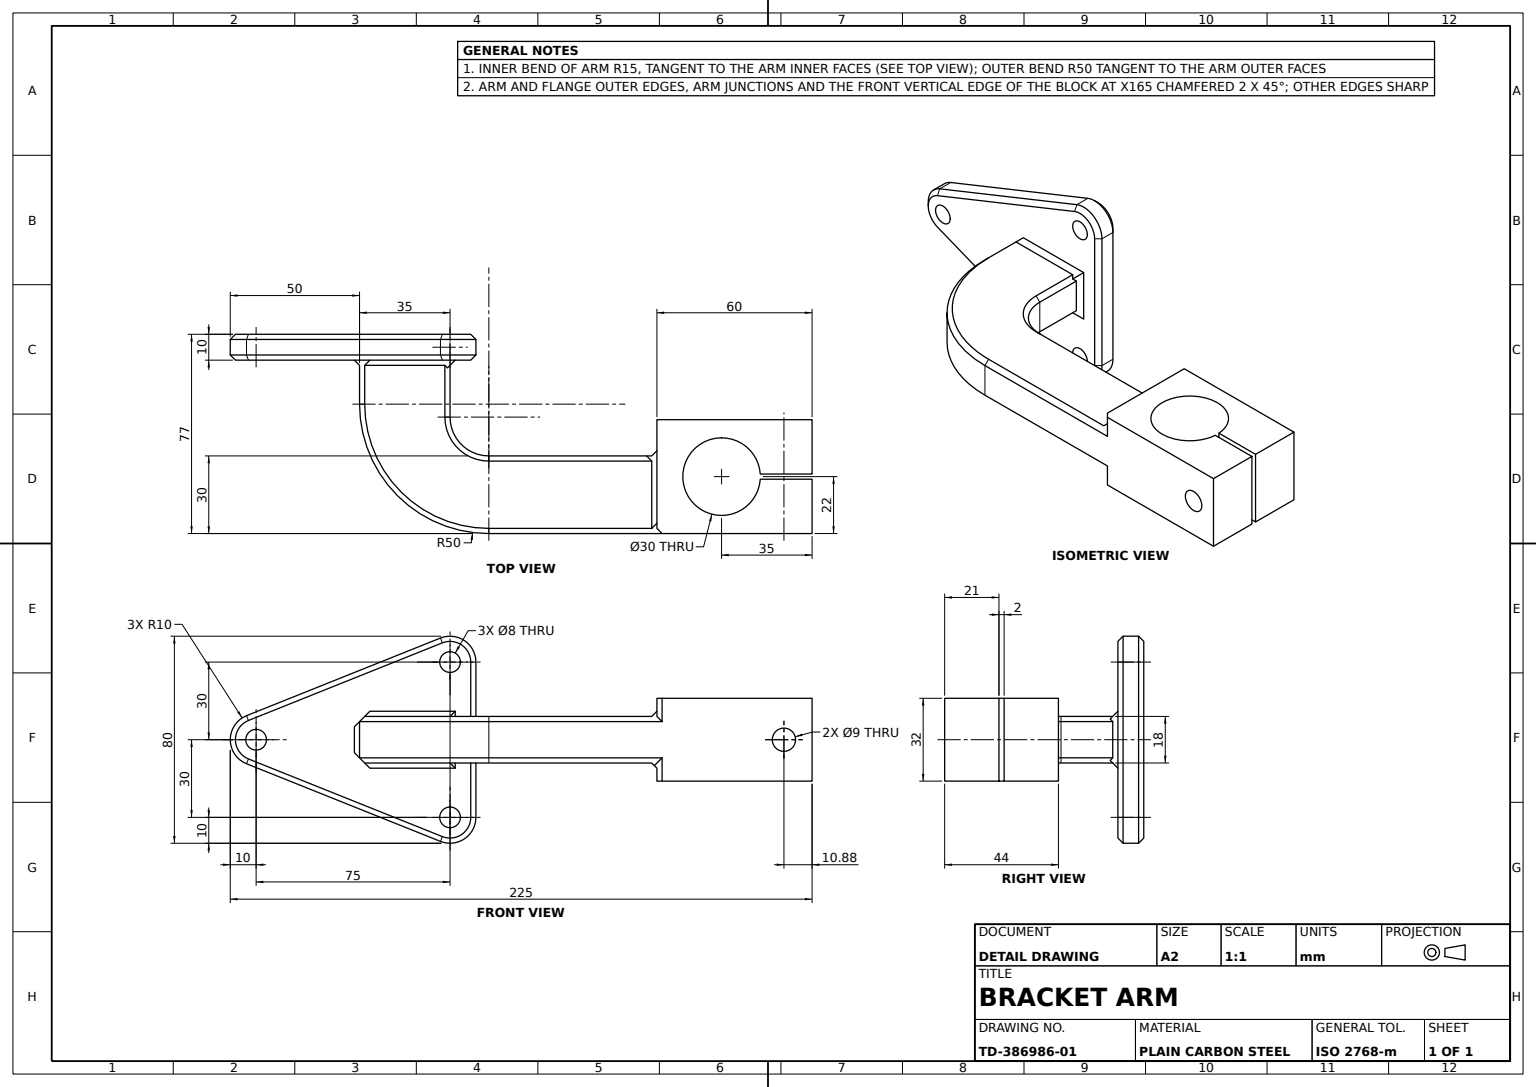
SolidWorks part; units mm, degrees
material "Plain Carbon Steel"
ref_plane "Front Plane" through (0, 0, 0) normal (0, 0, 1) x (1, 0, 0)
ref_plane "Top Plane" through (0, 0, 0) normal (0, 1, 0) x (1, 0, 0)
ref_plane "Right Plane" through (0, 0, 0) normal (1, 0, 0) x (0, 0, -1)
sketch "Clamp Block Sketch" plane through (0, 0, 0) normal (0, 0, 1) x (1, 0, 0)
  line L0 (0, 0) -> (60, 0)
  line L1 (60, 0) -> (60, -32)
  line L2 (60, -32) -> (0, -32)
  line L3 (0, -32) -> (0, 0)
  dimension "D1" = 60
  dimension "D2" = 32
extrude "Clamp Block" add sketch "Clamp Block Sketch" against normal blind 44
sketch "Split Bore Sketch" plane through (0, -32, 0) normal (0, -1, 0) x (1, 0, 0)
  line L0 (60, -44) -> (60, 0) construction
  line L1 (0, 0) -> (60, 0) construction
  line L2 (60, -21) -> (60, -23)
  line L3 (60, -21) -> (39.9666, -21)
  line L5 (39.9666, -23) -> (60, -23)
  arc A0 (39.9666, -21) -> (39.9666, -23) centre (25, -22) ccw
  dimension "D1" = 30
  dimension "D2" = 35
  dimension "D3" = 22
  dimension "D4" = 20.0334
  dimension "D5" = 2
extrude "Split Bore Cut" cut sketch "Split Bore Sketch" against normal blind 44
sketch "Clamp Bolt Hole Sketch" plane through (0, 0, 0) normal (0, 0, 1) x (1, 0, 0)
  line L0 (60, 0) -> (0, 0) construction
  line L1 (60, -32) -> (60, 0) construction
  circle A0 centre (49.1198, -16) radius 4.5
  dimension "D1" = 9
  dimension "D2" = 16
  dimension "D3" = 10.8802
extrude "Clamp Bolt Hole" cut sketch "Clamp Bolt Hole Sketch" against normal blind 60
sketch "Arm Sketch" plane through (0, 0, 0) normal (-1, 0, 0) x (0, 0, 1)
  line L1 (0, 0) -> (0, -32) construction
  line L2 (0, -7) -> (-30, -7)
  line L3 (-30, -7) -> (-30, -25)
  line L4 (-30, -25) -> (0, -25)
  line L6 (0, -7) -> (0, -25)
  line L7 (-44, 0) -> (0, 0) construction
  dimension "D1" = 7
  dimension "D2" = 30
  dimension "D3" = 18
extrude "Arm" add sketch "Arm Sketch" along normal blind 65
sketch "Arm Bend Sketch" plane through (0, -25, 0) normal (0, -1, 0) x (1, 0, 0)
  line L0 (-115, -67) -> (-80, -67)
  line L1 (-80, -67) -> (-80, -45)
  line L2 (-65, 0) -> (0, 0) construction
  line L3 (-65, -30) -> (-65, 0) construction
  line L4 (-65, -30) -> (0, -30) construction
  line L5 (-115, -67) -> (-115, -50)
  line L6 (-65, 0) -> (-65, -30)
  arc A0 (-115, -50) -> (-65, 0) centre (-65, -50) cw
  arc A1 (-80, -45) -> (-65, -30) centre (-65, -45) cw
  dimension "D3" = 50
  dimension "D1" = 35
  dimension "D2" = 22
extrude "Arm Bend" add sketch "Arm Bend Sketch" against normal blind 18
sketch "Mounting Flange Sketch" plane through (0, 0, -67) normal (0, 0, -1) x (-1, 0, 0)
  line L0 (115, -7) -> (115, -25) construction
  line L1 (115, -25) -> (80, -25) construction
  line L4 (83.7139, 23.2848) -> (158.7139, -6.7152)
  line L5 (83.7139, -55.2848) -> (158.7139, -25.2848)
  line L6 (70, 14) -> (70, -46)
  arc A0 (83.7139, 23.2848) -> (70, 14) centre (80, 14) ccw
  arc A1 (70, -46) -> (83.7139, -55.2848) centre (80, -46) ccw
  arc A2 (158.7139, -25.2848) -> (158.7139, -6.7152) centre (155, -16) ccw
  dimension "D4" = 10
  dimension "D5" = 10
  dimension "D6" = 10
  dimension "D1" = 40
  dimension "D2" = 43.7139
  dimension "D3" = 31.2861
  dimension "D7" = 9
extrude "Mounting Flange" add sketch "Mounting Flange Sketch" along normal blind 10
sketch "Flange Holes Sketch" plane through (0, 0, -77) normal (0, 0, -1) x (-1, 0, 0)
  circle A0 centre (80, 14) radius 4
  circle A1 centre (155, -16) radius 4
  circle A2 centre (80, -46) radius 4
  dimension "D1" = 8
  dimension "D2" = 8
  dimension "D3" = 8
extrude "Flange Holes 3xØ8" cut sketch "Flange Holes Sketch" against normal blind 10
chamfer "Arm-Bend Chamfer" distance 2 angle 45 3 edges at (-115, -25, -58.5) (-100.3553, -25, -14.6447) (-32.5, -25, 0)
chamfer "Clamp Block Chamfer A" distance 2 angle 45 1 edges at (0, -27.5, 0)
chamfer "Arm-Clamp Chamfer A" distance 2 angle 45 1 edges at (0, -25, -16)
chamfer "Arm Edge Chamfer" distance 2 angle 45 3 edges at (-115, -7, -58.5) (-100.3553, -7, -14.6447) (-32.5, -7, 0)
chamfer "Arm-Clamp Chamfer B" distance 2 angle 45 1 edges at (0, -7, -16)
chamfer "Clamp Block Chamfer B" distance 2 angle 45 1 edges at (0, -4.5, 0)
chamfer "Arm-Flange Chamfer A" distance 2 angle 45 7 edges at (-70, -16, -67) (-74.3937, 22.2807, -67) (-121.2139, 8.2848, -67) (-74.3937, -54.2807, -67) (-165, -16, -67) (-121.2139, -40.2848, -67) (-96.5, -25, -67)
chamfer "Bend-Flange Chamfer A" distance 2 angle 45 1 edges at (-115, -16, -67)
chamfer "Arm-Flange Chamfer B" distance 2 angle 45 1 edges at (-96.5, -7, -67)
chamfer "Bend-Flange Chamfer B" distance 2 angle 45 1 edges at (-80, -16, -67)
chamfer "Flange Edge Chamfer" distance 2 angle 45 6 edges at (-74.3937, -54.2807, -77) (-121.2139, -40.2848, -77) (-70, -16, -77) (-165, -16, -77) (-74.3937, 22.2807, -77) (-121.2139, 8.2848, -77)
chamfer "Bend Edge Chamfer A" distance 2 angle 45 3 edges at (-33.5, -25, -30) (-75.6066, -25, -34.3934) (-80, -25, -55)
chamfer "Bend Edge Chamfer B" distance 2 angle 45 3 edges at (-33.5, -7, -30) (-75.6066, -7, -34.3934) (-80, -7, -55)
chamfer "Arm-Clamp Chamfer C" distance 2 angle 45 1 edges at (0, -16, -30)
